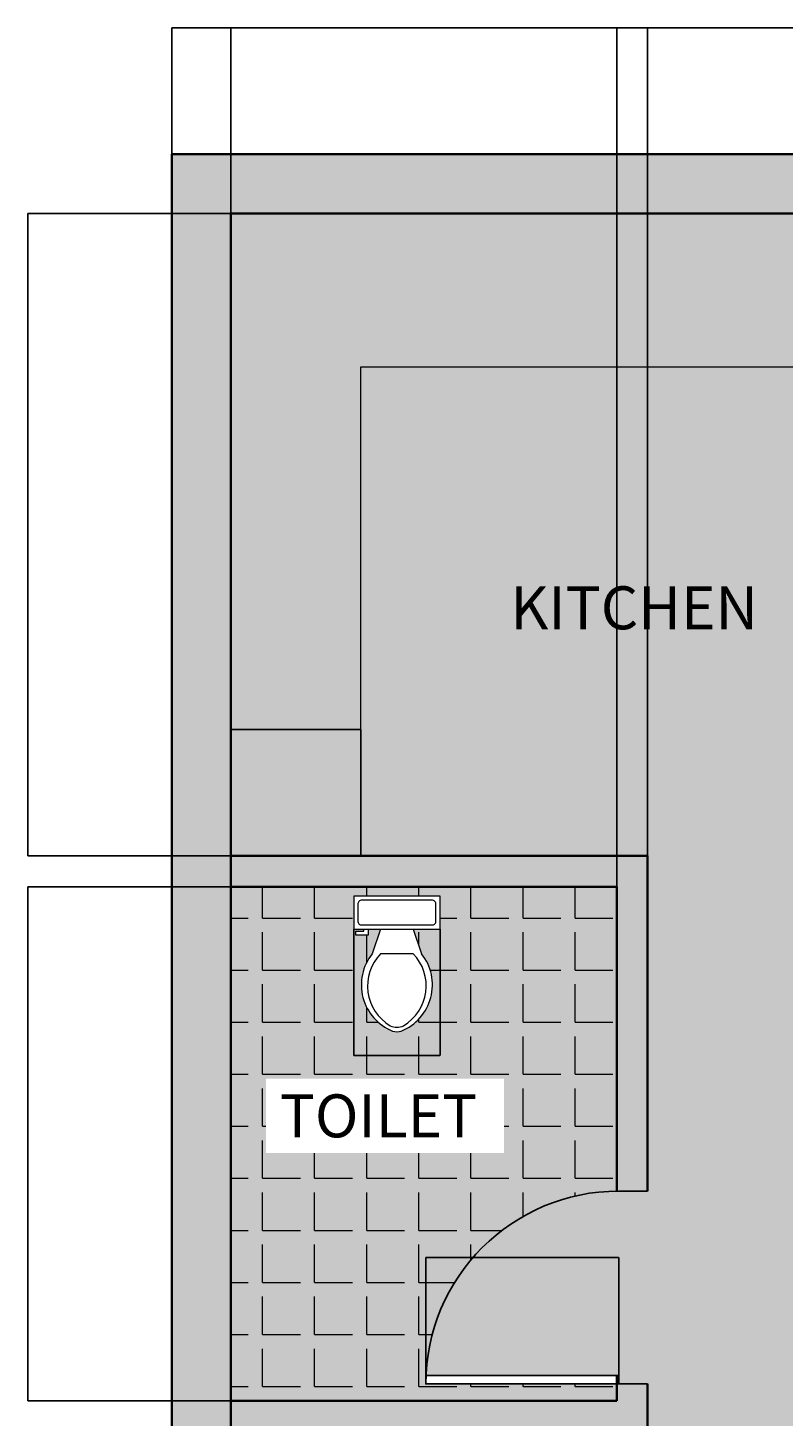
# Model space of a CAD drawing. Units: millimetres. Extents: x 1166 to 16630, y -7192 to 2820.
# Tile 5 of 8: x 1166 to 4103, y -2583 to 2820. Entities that reach past the tile are written whole.
import ezdxf

# ---------------------------------------------------------------- set-up
doc = ezdxf.new("R2010")
doc.units = ezdxf.units.MM
for name, color, linetype, lineweight in [('A-ANNO-DIMS', 2, 'Continuous', 18), ('A-AREA-IDEN', 7, 'Continuous', 18), ('A-DOOR', 4, 'Continuous', 25), ('A-FLOR-CASE', 8, 'Continuous', 18), ('A-FLOR-FIXT', 8, 'Continuous', 18), ('A-FLOR-PATT', 8, 'Continuous', 13), ('A-WALL', 7, 'Continuous', 35)]:
    doc.layers.add(name, color=color, linetype=linetype, lineweight=lineweight)
for name, color, linetype, lineweight, true_color in [('A-FLOR-CASE-PATT', 9, 'Continuous', 13, 0xc7c8ca), ('A-FLOR-FNSH-PATT', 254, 'Continuous', 13, 0xfeeab9), ('A-WALL-PATT', 254, 'Continuous', 13, 0xcecce6)]:
    doc.layers.add(name, color=color, linetype=linetype, lineweight=lineweight, true_color=true_color)
doc.styles.get("Standard").update_dxf_attribs({"font": 'arial.ttf'})
doc.dimstyles.get("Standard").update_dxf_attribs({"dimtxt": 0.18, "dimasz": 0.18, "dimexe": 0.18, "dimexo": 0.0625, "dimgap": 0.09, "dimtad": 0, "dimtih": 1, "dimtoh": 1, "dimdec": 4, "dimzin": 0, "dimdsep": 46, "dimtxsty": 'Standard', "dimcen": 0.09, "dimadec": 0, "dimazin": 0, "dimtfac": 1, "dimtdec": 4, "dimtofl": 0, "dimtmove": 0, "dimatfit": 3, "dimfxl": 1, "dimtolj": 1, "dimtzin": 0, "dimarcsym": 0})

# ---------------------------------------------------------------- blocks, each defined once
blk = doc.blocks.new('*U3')
for p, q in [((0, 0), (0, -6)), ((40, 0), (40, -6))]:
    blk.add_line(p, q)
blk.add_lwpolyline([(0, 0), (0, 40), (1.75, 40), (1.75, 0)], close=True)
blk.add_arc((0, 0), 40, 0, 90)
blk = doc.blocks.new('*U8')
for p, q in [((9.5, -6), (9.5, -2)), ((-10, -8.5), (-8, -8.5)), ((-10, -9.5), (-10, -8.5)), ((-7, -9.5), (-10, -9.5)), ((-8, -8.5), (-8, -8)), ((-7, -8), (-7, -9.5)), ((-4, -8), (-6, -14)), ((4, -8), (6, -14)), ((4, -14), (-4, -14))]:
    blk.add_line(p, q)
blk.add_lwpolyline([(10.5, -8), (10.5, 0), (-10.5, 0), (-10.5, -8)], close=True)
for points in [[(-9.5, -2), (-9.5, -6)], [(8.5, -1), (-8.5, -1)], [(-8.5, -7), (8.5, -7)]]:
    blk.add_lwpolyline(points)
for centre, radius, start, end in [((-8.62, -1.88), 0.884, 81.8699, 188.1301), ((8.62, -1.88), 0.884, 351.8699, 98.1301), ((-8.62, -6.12), 0.884, 171.8699, 278.1301), ((8.62, -6.12), 0.884, 261.8699, 8.1301), ((3.52, -21.58), 12.17, 141.4691, 247.9714), ((4.2, -21.82), 11.33, 136.3677, 238.9468), ((-3.52, -21.58), 12.17, 292.0284, 38.5307), ((-4.2, -21.82), 11.33, 301.053, 43.6321), ((0, -27.88), 4, 245.7318, 294.2682), ((0, -29), 4, 254.8605, 285.1395)]:
    blk.add_arc(centre, radius, start, end)
blk = doc.blocks.new('*D23')
at = {"layer": 'A-ANNO-DIMS', "color": 0, "lineweight": -2, "transparency": 16777216}
for p, q in [((1725.9, 2327.5), (1725.9, 2819.6)), ((1726.1, 2819.5), (4725.6, 2819.5)), ((7725.8, 2819.5), (4726.3, 2819.5)), ((7725.9, 2327.5), (7725.9, 2819.6))]:
    blk.add_line(p, q, dxfattribs=at)
at = {"layer": 'A-ANNO-DIMS', "color": 0, "transparency": 16777216}
for points in [[(1726.1, 2819.5), (1726.1, 2819.4), (1725.9, 2819.5)], [(7725.8, 2819.5), (7725.8, 2819.4), (7725.9, 2819.5)]]:
    blk.add_solid(points, dxfattribs=at)
at = {"layer": 'Defpoints', "color": 0, "transparency": 16777216}
for p in [(7725.9, 2819.5), (1725.9, 2327.5), (7725.9, 2327.5)]:
    blk.add_point(p, dxfattribs=at)
at = {"layer": 'A-ANNO-DIMS', "color": 0, "transparency": 16777216, "insert": (4725.9, 2819.5), "char_height": 0.18, "attachment_point": 5}
blk.add_mtext('\\A1;6000', dxfattribs=at)
blk = doc.blocks.new('*D25')
at = {"layer": 'A-ANNO-DIMS', "color": 0, "lineweight": -2, "transparency": 16777216}
for p, q in [((1955.939441, 2097.524735), (1955.939441, 2819.642235)), ((1956.119441, 2819.462235), (3310.579441, 2819.462235)), ((4665.759441, 2819.462235), (3311.299441, 2819.462235)), ((4665.939441, 2097.524735), (4665.939441, 2819.642235))]:
    blk.add_line(p, q, dxfattribs=at)
at = {"layer": 'A-ANNO-DIMS', "color": 0, "transparency": 16777216}
for points in [[(1956.119441, 2819.492235), (1956.119441, 2819.432235), (1955.939441, 2819.462235)], [(4665.759441, 2819.492235), (4665.759441, 2819.432235), (4665.939441, 2819.462235)]]:
    blk.add_solid(points, dxfattribs=at)
at = {"layer": 'Defpoints', "color": 0, "transparency": 16777216}
for p in [(4665.939441, 2819.462235), (1955.939441, 2097.462235), (4665.939441, 2097.462235)]:
    blk.add_point(p, dxfattribs=at)
at = {"layer": 'A-ANNO-DIMS', "color": 0, "transparency": 16777216, "insert": (3310.939441, 2819.462235), "char_height": 0.18, "attachment_point": 5}
blk.add_mtext('\\A1;2710', dxfattribs=at)
blk = doc.blocks.new('*D27')
at = {"layer": 'A-ANNO-DIMS', "color": 0, "lineweight": -2, "transparency": 16777216}
for p, q in [((1955.9, 2097.5), (1165.9, 2097.5)), ((1166.1, 2097.3), (1166.1, 847.6)), ((1166.1, -402.4), (1166.1, 847.3)), ((1955.9, -402.5), (1165.9, -402.5))]:
    blk.add_line(p, q, dxfattribs=at)
at = {"layer": 'A-ANNO-DIMS', "color": 0, "transparency": 16777216}
for points in [[(1166.1, 2097.3), (1166.1, 2097.3), (1166.1, 2097.5)], [(1166.1, -402.4), (1166.1, -402.4), (1166.1, -402.5)]]:
    blk.add_solid(points, dxfattribs=at)
at = {"layer": 'Defpoints', "color": 0, "transparency": 16777216}
for p in [(1166.1, 2097.5), (1955.9, 2097.5), (1955.9, -402.5)]:
    blk.add_point(p, dxfattribs=at)
at = {"layer": 'A-ANNO-DIMS', "color": 0, "transparency": 16777216, "insert": (1166.1, 847.5), "char_height": 0.18, "attachment_point": 5}
blk.add_mtext('\\A1;2500', dxfattribs=at)
blk = doc.blocks.new('*D28')
at = {"layer": 'A-ANNO-DIMS', "color": 0, "lineweight": -2, "transparency": 16777216}
for p, q in [((1955.9, -522.5), (1955.9, 2819.6)), ((1956.1, 2819.5), (2705.6, 2819.5)), ((3455.8, 2819.5), (2706.3, 2819.5)), ((3455.9, -522.5), (3455.9, 2819.6))]:
    blk.add_line(p, q, dxfattribs=at)
at = {"layer": 'A-ANNO-DIMS', "color": 0, "transparency": 16777216}
for points in [[(1956.1, 2819.5), (1956.1, 2819.4), (1955.9, 2819.5)], [(3455.8, 2819.5), (3455.8, 2819.4), (3455.9, 2819.5)]]:
    blk.add_solid(points, dxfattribs=at)
at = {"layer": 'Defpoints', "color": 0, "transparency": 16777216}
for p in [(3455.9, 2819.5), (1955.9, -522.5), (3455.9, -522.5)]:
    blk.add_point(p, dxfattribs=at)
at = {"layer": 'A-ANNO-DIMS', "color": 0, "transparency": 16777216, "insert": (2705.9, 2819.5), "char_height": 0.18, "attachment_point": 5}
blk.add_mtext('\\A1;1500', dxfattribs=at)
blk = doc.blocks.new('*D29')
at = {"layer": 'A-ANNO-DIMS', "color": 0, "lineweight": -2, "transparency": 16777216}
for p, q in [((1955.9, -522.5), (1165.9, -522.5)), ((1166.1, -522.7), (1166.1, -1522.4)), ((1166.1, -2522.4), (1166.1, -1522.7)), ((1955.9, -2522.5), (1165.9, -2522.5))]:
    blk.add_line(p, q, dxfattribs=at)
at = {"layer": 'A-ANNO-DIMS', "color": 0, "transparency": 16777216}
for points in [[(1166.1, -522.7), (1166.1, -522.7), (1166.1, -522.5)], [(1166.1, -2522.4), (1166.1, -2522.4), (1166.1, -2522.5)]]:
    blk.add_solid(points, dxfattribs=at)
at = {"layer": 'Defpoints', "color": 0, "transparency": 16777216}
for p in [(1955.9, -522.5), (1166.1, -2522.5), (1955.9, -2522.5)]:
    blk.add_point(p, dxfattribs=at)
at = {"layer": 'A-ANNO-DIMS', "color": 0, "transparency": 16777216, "insert": (1166.1, -1522.5), "char_height": 0.18, "attachment_point": 5}
blk.add_mtext('\\A1;2000', dxfattribs=at)
blk = doc.blocks.new('*D35')
at = {"layer": 'A-ANNO-DIMS', "color": 0, "lineweight": -2, "transparency": 16777216}
for p, q in [((2713.4, -2456.6), (2713.4, -1964.5)), ((2713.6, -1964.6), (3088.2, -1964.6)), ((3463.3, -1964.6), (3088.7, -1964.6)), ((3463.4, -2456.6), (3463.4, -1964.5))]:
    blk.add_line(p, q, dxfattribs=at)
at = {"layer": 'A-ANNO-DIMS', "color": 0, "transparency": 16777216}
for points in [[(2713.6, -1964.6), (2713.6, -1964.7), (2713.4, -1964.6)], [(3463.3, -1964.6), (3463.3, -1964.7), (3463.4, -1964.6)]]:
    blk.add_solid(points, dxfattribs=at)
at = {"layer": 'Defpoints', "color": 0, "transparency": 16777216}
for p in [(3463.4, -1964.6), (2713.4, -2456.6), (3463.4, -2456.6)]:
    blk.add_point(p, dxfattribs=at)
at = {"layer": 'A-ANNO-DIMS', "color": 0, "transparency": 16777216, "insert": (3088.4, -1964.6), "char_height": 0.18, "attachment_point": 5}
blk.add_mtext('\\A1;750', dxfattribs=at)
blk = doc.blocks.new('*D37')
at = {"layer": 'A-ANNO-DIMS', "color": 0, "lineweight": -2, "transparency": 16777216}
for p, q in [((3455.9, -1706.6), (3455.9, 2819.6)), ((3456.1, 2819.5), (3515.7, 2819.5)), ((3575.8, 2819.5), (3516.2, 2819.5)), ((3575.9, -1706.6), (3575.9, 2819.6))]:
    blk.add_line(p, q, dxfattribs=at)
at = {"layer": 'A-ANNO-DIMS', "color": 0, "transparency": 16777216}
for points in [[(3456.1, 2819.5), (3456.1, 2819.4), (3455.9, 2819.5)], [(3575.8, 2819.5), (3575.8, 2819.4), (3575.9, 2819.5)]]:
    blk.add_solid(points, dxfattribs=at)
at = {"layer": 'Defpoints', "color": 0, "transparency": 16777216}
for p in [(3575.9, 2819.5), (3455.9, -1706.7), (3575.9, -1706.6)]:
    blk.add_point(p, dxfattribs=at)
at = {"layer": 'A-ANNO-DIMS', "color": 0, "transparency": 16777216, "insert": (3515.9, 2819.5), "char_height": 0.18, "attachment_point": 5}
blk.add_mtext('\\A1;120', dxfattribs=at)
blk = doc.blocks.new('*D41')
at = {"layer": 'A-ANNO-DIMS', "color": 0, "lineweight": -2, "transparency": 16777216}
for p, q in [((1955.9, -402.5), (1955.9, 89.6)), ((1956.1, 89.5), (2207.8, 89.5)), ((2460.4, 89.5), (2208.6, 89.5)), ((2460.5, -402.5), (2460.5, 89.6))]:
    blk.add_line(p, q, dxfattribs=at)
at = {"layer": 'A-ANNO-DIMS', "color": 0, "transparency": 16777216}
for points in [[(1956.1, 89.5), (1956.1, 89.4), (1955.9, 89.5)], [(2460.4, 89.5), (2460.4, 89.4), (2460.5, 89.5)]]:
    blk.add_solid(points, dxfattribs=at)
at = {"layer": 'Defpoints', "color": 0, "transparency": 16777216}
for p in [(2460.5, 89.5), (1955.9, -402.5), (2460.5, -402.5)]:
    blk.add_point(p, dxfattribs=at)
at = {"layer": 'A-ANNO-DIMS', "color": 0, "transparency": 16777216, "insert": (2208.2, 89.5), "char_height": 0.18, "attachment_point": 5}
blk.add_mtext('\\A1;504.6', dxfattribs=at)
blk = doc.blocks.new('*D43')
at = {"layer": 'A-ANNO-DIMS', "color": 0, "lineweight": -2, "transparency": 16777216}
for p, q in [((2433.1, -687.1), (2433.1, -1179.2)), ((2768.8, -687.1), (2768.8, -1179.2)), ((2433.3, -1179), (2600.5, -1179)), ((2768.6, -1179), (2601.4, -1179))]:
    blk.add_line(p, q, dxfattribs=at)
at = {"layer": 'A-ANNO-DIMS', "color": 0, "transparency": 16777216}
for points in [[(2433.3, -1179), (2433.3, -1179.1), (2433.1, -1179)], [(2768.6, -1179), (2768.6, -1179.1), (2768.8, -1179)]]:
    blk.add_solid(points, dxfattribs=at)
at = {"layer": 'Defpoints', "color": 0, "transparency": 16777216}
for p in [(2433.1, -687), (2768.8, -687), (2433.1, -1179)]:
    blk.add_point(p, dxfattribs=at)
at = {"layer": 'A-ANNO-DIMS', "color": 0, "transparency": 16777216, "insert": (2601, -1179), "char_height": 0.18, "attachment_point": 5}
blk.add_mtext('\\A1;335.66', dxfattribs=at)

msp = doc.modelspace()

# ---------------------------------------------------------------- hatches: boundary and pattern name
at = {"layer": 'A-FLOR-CASE-PATT'}
h = msp.add_hatch(color=256, dxfattribs=at)
h.dxf.hatch_style = 1
h.paths.add_polyline_path([(2460.545, 1500.697), (4665.939, 1500.697), (4665.939, 2097.462), (1955.939, 2097.462), (1955.939, -402.538), (2460.545, -402.538)])
at = {"layer": 'A-FLOR-FNSH-PATT', "transparency": 33554523}
h = msp.add_hatch(color=256, dxfattribs=at)
h.dxf.hatch_style = 1
h.paths.add_polyline_path([(7725.939, 2327.462), (1725.939, 2327.462), (1725.939, -5672.538), (5309.615, -5672.538), (5309.615, -2642.538), (5189.615, -2642.538), (5189.615, -5442.538), (1955.939, -5442.538), (1955.939, 2097.462), (4665.939, 2097.462), (4665.939, 150.2), (4815.939, 150.2, -0.40145271), (5814.982, -806.05), (5815.939, -806.05), (5815.939, -849.8), (4815.939, -849.8), (4785.939, -849.8), (4785.939, -902.538), (7495.939, -902.538), (7495.939, -2522.538), (4884.014, -2522.538), (4884.014, -2642.538), (7725.939, -2642.538)], flags=17)
h.paths.add_polyline_path([(6066.077, 618.421), (6066.077, 1624.186), (7407.098, 1624.186), (7407.098, 618.421)], flags=16)
h.paths.add_polyline_path([(4979.212, 660.219), (4799.278, 660.219), (4799.278, 780.174), (4789.282, 790.171), (4789.282, 870.141), (4799.278, 880.137), (4799.278, 1259.997), (4979.212, 1259.997), (4979.212, 1230.008), (4989.208, 1230.008), (4989.208, 1110.052), (4979.212, 1110.052), (4979.212, 1100.056), (4989.208, 1100.056), (4989.208, 980.1), (4979.212, 980.1), (4979.212, 950.111), (4989.208, 950.111), (4989.208, 940.115, -0.09090909), (4989.208, 720.196), (4989.208, 710.2), (4979.212, 710.2)], flags=16)
h.paths.add_polyline_path([(4974.214, 665.217), (4804.276, 665.217), (4804.276, 1254.999), (4974.214, 1254.999)], flags=0)
h.paths.add_polyline_path([(6910.92, 618.421), (6910.92, 873.215), (7165.714, 873.215), (7165.714, 1490.084), (7386.983, 1490.084), (7386.983, 1141.419), (7165.714, 1141.419), (7165.714, 1101.188), (7386.983, 1101.188), (7386.983, 752.523), (7132.189, 752.523), (7132.189, 839.689)], flags=16)
h.paths.add_polyline_path([(4815.939, 150.2), (4665.939, 150.2), (4665.939, 1500.697), (2460.545, 1500.697), (2460.545, -402.538), (3575.939, -402.538), (3575.939, -1706.64), (3463.439, -1706.64, 0.40145271), (2714.158, -2423.828), (3463.439, -2423.828), (3463.439, -2456.64), (3455.939, -2522.538), (3455.939, -2456.64), (2713.439, -2456.64), (2713.439, -2423.828), (2714.158, -2423.828, -0.39855266), (3455.939, -1706.678), (3455.939, -1706.64), (3575.939, -1706.64), (3575.939, -402.538), (2460.545, -402.538), (2460.545, 1500.697), (4665.939, 1500.697), (4665.939, 150.2), (4785.939, 150.2), (4785.939, 2097.462), (7495.939, 2097.462), (7495.939, -2522.538), (4884.014, -2522.538), (4884.014, -2642.538), (7725.939, -2642.538), (7725.939, 2327.462), (1725.939, 2327.462), (1725.939, -5672.538), (5309.615, -5672.538), (5309.615, -2642.538), (4884.014, -2642.538), (4884.014, -2522.538), (4884.014, -1822.538), (4665.939, -1822.538), (4665.939, -1722.538), (4665.939, -1022.538), (4665.939, -849.8), (4815.939, -849.8), (4815.939, -806.05), (5814.982, -806.05, 0.40145271)])
h.paths.add_polyline_path([(1955.939, -4323.626), (1965.936, -4313.63), (1965.936, -3933.77), (2145.869, -3933.77), (2145.869, -3963.759), (2155.866, -3963.759), (2155.866, -4083.715), (2145.869, -4083.715), (2145.869, -4093.711), (2155.866, -4093.711), (2155.866, -4213.667), (2145.869, -4213.667), (2145.869, -4243.656), (2155.866, -4243.656), (2155.866, -4253.652, -0.09090909), (2155.866, -4473.571), (2155.866, -4483.567), (2145.869, -4483.567), (2145.869, -4533.549), (1965.936, -4533.549), (1965.936, -4413.593), (1955.939, -4403.597)], flags=16)
h.paths.add_polyline_path([(3017.672, -1268.685), (3017.672, -1558.932), (2092.538, -1558.932), (2092.538, -1268.685)], flags=16)
h.paths.add_polyline_path([(2768.799, -687.028), (2664.904, -687.028), (2696.871, -782.93, -0.50132349), (2617.667, -1084.405, -0.13289091), (2584.271, -1084.405, -0.50131678), (2505.065, -782.933), (2537.033, -687.028), (2489.082, -687.028), (2489.082, -711.004), (2441.13, -711.004), (2441.13, -687.028), (2433.138, -687.028), (2433.138, -559.158), (2768.799, -559.158)], flags=16)
h.paths.add_polyline_path([(2752.815, -655.061, -0.41421356), (2740.827, -671.045), (2465.106, -671.045, -0.41421356), (2449.122, -659.057), (2449.122, -591.126, -0.41421356), (2461.11, -575.142), (2736.831, -575.142, -0.41421356), (2752.815, -587.13)], flags=0)
h.paths.add_polyline_path([(2627.247, -1063.016, -0.21500378), (2574.691, -1063.016, -0.48007965), (2537.034, -782.931), (2664.904, -782.931, -0.4800795)], flags=0)
h.paths.add_polyline_path([(4505.634, -3647.875), (4977.863, -3647.875, -0.19047621), (4977.864, -5173.541), (4505.634, -5173.541), (4505.634, -5064.565), (4533.929, -5064.565), (4533.929, -3756.851), (4505.634, -3756.851)], flags=16)
h.paths.add_polyline_path([(4880.114, -4192.756), (5003.372, -4192.756, -0.04962821), (5003.372, -4628.66), (4880.114, -4628.66)], flags=0)
h.paths.add_polyline_path([(2140.871, -3938.769), (2140.871, -4528.551), (1970.934, -4528.551), (1970.934, -3938.769)], flags=0)
h.paths.add_polyline_path([(7495.939, -1022.538), (6660.699, -1022.538), (6660.699, -1722.538, -0.21291191), (6697.901, -1739.132)], flags=16)
h.paths.add_polyline_path([(7495.939, -1022.538), (6697.901, -1739.132, -0.18498743), (6710.699, -1772.538), (7495.939, -1772.538)], flags=16)
h.paths.add_polyline_path([(7495.939, -1772.538), (6710.699, -1772.538, -0.18498743), (6697.901, -1805.944), (7495.939, -2522.538)], flags=16)
h.paths.add_polyline_path([(6697.901, -1805.944, -0.21291191), (6660.699, -1822.538), (6660.699, -2522.538), (7495.939, -2522.538)], flags=16)
h.paths.add_polyline_path([(6660.699, -1822.538), (6438.613, -1822.538), (6438.613, -2522.538), (6660.699, -2522.538)], flags=16)
h.paths.add_polyline_path([(6438.613, -1822.538), (6216.528, -1822.538), (6216.528, -2522.538), (6438.613, -2522.538)], flags=16)
h.paths.add_polyline_path([(6216.528, -1822.538), (5994.442, -1822.538), (5994.442, -2522.538), (6216.528, -2522.538)], flags=16)
h.paths.add_polyline_path([(5994.442, -1822.538), (5772.357, -1822.538), (5772.357, -2522.538), (5994.442, -2522.538)], flags=16)
h.paths.add_polyline_path([(5550.271, -1822.538), (5328.185, -1822.538), (5328.185, -2522.538), (5550.271, -2522.538)], flags=16)
h.paths.add_polyline_path([(5328.185, -1822.538), (5106.1, -1822.538), (5106.1, -2522.538), (5328.185, -2522.538)], flags=16)
h.paths.add_polyline_path([(5106.1, -1822.538), (4884.014, -1822.538), (4884.014, -2522.538), (5106.1, -2522.538)], flags=16)
h.paths.add_polyline_path([(4884.014, -1022.538), (4665.939, -1022.538), (4665.939, -1722.538), (4884.014, -1722.538)], flags=16)
h.paths.add_polyline_path([(5106.1, -1022.538), (4884.014, -1022.538), (4884.014, -1722.538), (5106.1, -1722.538)], flags=16)
h.paths.add_polyline_path([(5550.271, -1022.538), (5328.185, -1022.538), (5328.185, -1722.538), (5550.271, -1722.538)], flags=16)
h.paths.add_polyline_path([(5328.185, -1022.538), (5106.1, -1022.538), (5106.1, -1722.538), (5328.185, -1722.538)], flags=16)
h.paths.add_polyline_path([(5772.357, -1022.538), (5550.271, -1022.538), (5550.271, -1722.538), (5772.357, -1722.538)], flags=16)
h.paths.add_polyline_path([(5994.442, -1022.538), (5772.357, -1022.538), (5772.357, -1722.538), (5994.442, -1722.538)], flags=16)
h.paths.add_polyline_path([(6216.528, -1022.538), (5994.442, -1022.538), (5994.442, -1722.538), (6216.528, -1722.538)], flags=16)
h.paths.add_polyline_path([(6660.699, -1022.538), (6438.613, -1022.538), (6438.613, -1722.538), (6660.699, -1722.538)], flags=16)
h.paths.add_polyline_path([(6438.613, -1022.538), (6216.528, -1022.538), (6216.528, -1722.538), (6438.613, -1722.538)], flags=16)
h.paths.add_polyline_path([(5772.357, -1822.538), (5550.271, -1822.538), (5550.271, -2522.538), (5772.357, -2522.538)], flags=16)
h.paths.add_polyline_path([(6660.699, -1722.538), (6438.613, -1722.538), (4665.939, -1722.538), (4665.939, -1822.538), (6660.699, -1822.538, 0.21291191), (6697.901, -1805.944, 0.64892437)], flags=16)
h.paths.add_polyline_path([(5860.25, -44.006), (7154.504, -44.006), (7154.504, 215.689), (5860.25, 215.689)], flags=24)
h.paths.add_polyline_path([(2102.336, -1543.656), (3007.075, -1543.656), (3007.075, -1283.961), (2102.336, -1283.961)], flags=8)
h.paths.add_polyline_path([(2887.503, -4248.68), (3740.372, -4248.68), (3740.372, -3989.156), (2887.503, -3989.156)], flags=24)
h.paths.add_polyline_path([(2999.436, 433.054), (4111.829, 433.054), (4111.829, 692.578), (2999.436, 692.578)], flags=24)
at = {"layer": 'A-FLOR-FNSH-PATT', "transparency": 33554590}
h = msp.add_hatch(color=256, dxfattribs=at)
h.dxf.hatch_style = 1
h.paths.add_polyline_path([(5309.615, -2642.538), (5309.615, -6304.141), (7725.939, -6304.141), (7725.939, -5672.538), (7725.939, -2642.538)])
edge = h.paths.add_edge_path(flags=16)
edge.add_ellipse((-448.972, -3645.43), major_axis=(-7430.723, 0), ratio=0.84230387, start_angle=182.1799503, end_angle=183.6504276, ccw=False)
edge.add_line((6974.174, -3362.862), (6984.716, -3362.862))
edge.add_ellipse((6982.281, -3380.397), major_axis=(-20.817, 0), ratio=0.84230387, start_angle=180, end_angle=270, ccw=False)
edge.add_line((7003.098, -3380.397), (7003.098, -3722.916))
edge.add_ellipse((6982.281, -3720.865), major_axis=(20.817, 0), ratio=0.84230387, start_angle=270, end_angle=360, ccw=False)
edge.add_ellipse((-142030.923, -3973.064), major_axis=(149013.204, 0), ratio=0.8423038695, start_angle=-0.38386678, end_angle=0.09022909, ccw=False)
edge.add_line((6977.567, -4971.397), (6984.47, -4971.397))
edge.add_ellipse((6982.281, -4988.932), major_axis=(20.817, 0), ratio=0.84230387, start_angle=0, end_angle=90, ccw=False)
edge.add_line((7003.098, -4988.932), (7003.098, -5331.243))
edge.add_ellipse((6982.281, -5329.4), major_axis=(-20.817, 0), ratio=0.84230387, start_angle=90, end_angle=180, ccw=False)
edge.add_line((6982.281, -5346.934), (6973.354, -5346.934))
edge.add_ellipse((-142030.923, -3973.064), major_axis=(149013.204, 0), ratio=0.8423038695, start_angle=-0.6186432, end_angle=-0.52827147, ccw=False)
edge.add_ellipse((6960.189, -5606.903), major_axis=(-31.226, 0), ratio=0.84230387, start_angle=179.371763, end_angle=248.464757, ccw=False)
edge.add_ellipse((-142041.332, -3973.064), major_axis=(-149045.372, 0), ratio=0.8423038661, start_angle=179.35344592, end_angle=179.3717628, ccw=False)
edge.add_ellipse((6916.87, -5654.054), major_axis=(-73.802, 0), ratio=0.84230387, start_angle=90, end_angle=179.353446, ccw=False)
edge.add_line((6916.87, -5716.218), (5995.23, -5716.218))
edge.add_ellipse((5995.23, -5654.054), major_axis=(73.802, 0), ratio=0.84230387, start_angle=180.646554, end_angle=270, ccw=False)
edge.add_ellipse((154953.432, -3973.064), major_axis=(-149045.372, 0), ratio=0.8423038697, start_angle=0.62823722, end_angle=0.6465541, ccw=False)
edge.add_ellipse((5951.911, -5606.903), major_axis=(31.226, 0), ratio=0.84230387, start_angle=111.535244, end_angle=180.628237, ccw=False)
edge.add_ellipse((154943.023, -3973.064), major_axis=(-149013.204, 0), ratio=0.8423038695, start_angle=0.52827147, end_angle=0.6465541, ccw=False)
edge.add_line((5938.746, -5346.934), (5927.384, -5346.934))
edge.add_ellipse((5929.819, -5329.4), major_axis=(20.817, 0), ratio=0.84230387, start_angle=180, end_angle=270, ccw=False)
edge.add_line((5909.002, -5329.4), (5909.002, -4986.881))
edge.add_ellipse((5929.819, -4988.932), major_axis=(-20.817, 0), ratio=0.84230387, start_angle=-90, end_angle=0, ccw=False)
edge.add_line((5929.819, -4971.397), (5934.533, -4971.397))
edge.add_ellipse((154943.023, -3973.064), major_axis=(-149013.204, 0), ratio=0.8423038695, start_angle=-0.09022909, end_angle=0.38386678, ccw=False)
edge.add_ellipse((5929.819, -3720.865), major_axis=(-20.817, 0), ratio=0.84230387, start_angle=0, end_angle=90, ccw=False)
edge.add_line((5909.002, -3720.865), (5909.002, -3378.346))
edge.add_ellipse((5929.819, -3380.397), major_axis=(20.817, 0), ratio=0.84230387, start_angle=90, end_angle=180, ccw=False)
edge.add_line((5929.819, -3362.862), (5937.926, -3362.862))
edge.add_ellipse((13361.072, -3645.43), major_axis=(7430.723, 0), ratio=0.84230387, start_angle=176.3495724, end_angle=177.8200497, ccw=False)
edge.add_ellipse((6843.239, -6808.261), major_axis=(4407.333, 0), ratio=0.84230387, start_angle=102.125966, end_angle=103.780529, ccw=False)
edge.add_ellipse((6843.239, -6711.831), major_axis=(4294.728, 0), ratio=0.84230387, start_angle=100.209539, end_angle=102.444627, ccw=False)
edge.add_ellipse((5718.978, -189.342), major_axis=(-3530.283, 0), ratio=0.84230387, start_angle=99.256566, end_angle=102.554933)
edge.add_line((6369.843, -3111.939), (6452.047, -3066.483))
edge.add_ellipse((6456.05, -3074.757), major_axis=(-10.409, 0), ratio=0.84230387, start_angle=270, end_angle=307.93313, ccw=False)
edge.add_ellipse((6456.05, -3074.757), major_axis=(-10.409, 0), ratio=0.84230387, start_angle=232.06687, end_angle=270, ccw=False)
edge.add_line((6461.762, -3067.428), (6542.257, -3111.939))
edge.add_ellipse((7193.122, -189.342), major_axis=(3530.283, 0), ratio=0.84230387, start_angle=257.445067, end_angle=260.743434)
edge.add_ellipse((6068.861, -6711.831), major_axis=(4294.728, 0), ratio=0.84230387, start_angle=77.555373, end_angle=79.790461, ccw=False)
edge.add_ellipse((6068.861, -6808.261), major_axis=(-4407.333, 0), ratio=0.84230387, start_angle=256.219471, end_angle=257.874034, ccw=False)
edge = h.paths.add_edge_path(flags=0)
edge.add_ellipse((5799.636, -3484.806), major_axis=(790.133, 0), ratio=0.84230387, start_angle=0, end_angle=29.43857, ccw=False)
edge.add_line((6589.77, -3484.806), (6589.77, -3517.866))
edge.add_line((6589.77, -3517.866), (6615.397, -3517.866))
edge.add_ellipse((6612.95, -3526.633), major_axis=(10.409, 0), ratio=0.84230387, start_angle=45.519789, end_angle=90, ccw=False)
edge.add_line((6619.584, -3519.877), (6697.577, -3574.216))
edge.add_line((6697.577, -3574.216), (6697.577, -3782.552))
edge.add_ellipse((6643.673, -3780.461), major_axis=(5.016, 89.187), ratio=0.60383358, start_angle=106.342592, end_angle=270.997986, ccw=False)
edge.add_line((6589.77, -3793.028), (6589.77, -3484.806))
edge.add_ellipse((5799.636, -3484.806), major_axis=(790.133, 0), ratio=0.84230387, start_angle=0, end_angle=29.43857)
edge.add_ellipse((7112.464, -3484.806), major_axis=(-790.133, 0), ratio=0.84230387, start_angle=-29.43857, end_angle=0)
edge.add_line((6322.33, -3484.806), (6322.33, -3793.028))
edge.add_ellipse((6268.427, -3780.461), major_axis=(-5.016, 89.187), ratio=0.60383358, start_angle=89.002014, end_angle=253.657408, ccw=False)
edge.add_line((6214.523, -3782.552), (6214.523, -3574.216))
edge.add_line((6214.523, -3574.216), (6294.401, -3518.564))
edge.add_ellipse((6299.15, -3526.633), major_axis=(10.409, 0), ratio=0.84230387, start_angle=90, end_angle=134.480211, ccw=False)
edge.add_line((6299.15, -3517.866), (6322.33, -3517.866))
edge.add_line((6322.33, -3517.866), (6322.33, -3484.806))
edge.add_ellipse((7112.464, -3484.806), major_axis=(-790.133, 0), ratio=0.84230387, start_angle=-29.43857, end_angle=0, ccw=False)
edge = h.paths.add_edge_path(flags=0)
edge.add_line((6899.672, -4051.113), (6868.937, -4281.474))
edge.add_ellipse((6495.43, -5170.363), major_axis=(1119.455, 0), ratio=0.84230387, start_angle=67.208085, end_angle=85.12993)
edge.add_line((6575.565, -4229.86), (6336.535, -4229.86))
edge.add_ellipse((6416.67, -5170.363), major_axis=(1119.455, 0), ratio=0.84230387, start_angle=94.87007, end_angle=112.791915)
edge.add_line((6043.163, -4281.474), (6012.428, -4051.113))
edge.add_ellipse((6380.264, -4969.144), major_axis=(1150.303, 0), ratio=0.84230387, start_angle=94.277421, end_angle=111.834954, ccw=False)
edge.add_line((6307.939, -4002.156), (6604.161, -4002.156))
edge.add_ellipse((6531.836, -4969.144), major_axis=(-1150.303, 0), ratio=0.84230387, start_angle=248.165046, end_angle=265.722579, ccw=False)
edge = h.paths.add_edge_path(flags=0)
edge.add_ellipse((-142030.923, -3973.064), major_axis=(-148992.387, 0), ratio=0.8423038695, start_angle=179.62223581, end_angle=179.94440569, ccw=False)
edge.add_line((6956.9, -4955.389), (6903.068, -4744.03))
edge.add_ellipse((-45118.924, -4413.46), major_axis=(52023.473, 0), ratio=0.84230387, start_angle=-0.3640763, end_angle=0.1208974)
edge.add_line((6904.386, -4303.688), (6961.365, -4117.632))
edge = h.paths.add_edge_path(flags=0)
edge.add_line((5950.735, -4117.632), (6007.714, -4303.688))
edge.add_ellipse((58031.024, -4413.46), major_axis=(-52023.473, 0), ratio=0.84230387, start_angle=-0.1208974, end_angle=0.3640763)
edge.add_line((6009.031, -4744.03), (5955.2, -4955.389))
edge.add_ellipse((154943.023, -3973.064), major_axis=(-148992.387, 0), ratio=0.8423038696, start_angle=0.05559431, end_angle=0.37776419, ccw=False)
edge = h.paths.add_edge_path(flags=0)
edge.add_line((6868.937, -5013.198), (6868.937, -5277.993))
edge.add_ellipse((6456.05, -3571.079), major_axis=(2068.116, 0), ratio=0.84230387, start_angle=256.401865, end_angle=283.598135, ccw=False)
edge.add_line((6043.163, -5277.993), (6043.163, -5013.198))
edge.add_ellipse((6456.05, -3306.285), major_axis=(2068.116, 0), ratio=0.84230387, start_angle=256.401865, end_angle=283.598135)
edge = h.paths.add_edge_path(flags=0)
edge.add_ellipse((6827.303, -5415.313), major_axis=(-41.634, 0), ratio=0.84230387, start_angle=180, end_angle=270, ccw=False)
edge.add_line((6868.937, -5415.313), (6868.937, -5689.123))
edge.add_line((6868.937, -5689.123), (6043.163, -5689.123))
edge.add_line((6043.163, -5689.123), (6043.163, -5415.313))
edge.add_ellipse((6084.797, -5415.313), major_axis=(-41.634, 0), ratio=0.84230387, start_angle=-90, end_angle=0, ccw=False)
edge.add_line((6084.797, -5380.245), (6827.303, -5380.245))
h.paths.add_polyline_path([(3455.939, -522.538), (1955.939, -522.538), (1955.939, -2522.538), (3455.939, -2522.538), (3455.939, -2456.64), (2713.439, -2456.64), (2713.439, -2423.828), (2714.158, -2423.828, -0.39855266), (3455.939, -1706.678)])
h.paths.add_polyline_path([(2617.667, -1084.405, -0.13289091), (2584.271, -1084.405, -0.50131678), (2505.065, -782.933), (2537.033, -687.028), (2489.082, -687.028), (2489.082, -711.004), (2441.13, -711.004), (2441.13, -695.02), (2473.098, -695.02), (2473.098, -687.028), (2433.138, -687.028), (2433.138, -559.158), (2768.799, -559.158), (2768.799, -687.028), (2664.904, -687.028), (2696.871, -782.93, -0.50132349)], flags=16)
h.paths.add_polyline_path([(2627.247, -1063.016, -0.21500378), (2574.691, -1063.016, -0.48007965), (2537.034, -782.931), (2664.904, -782.931, -0.4800795)], flags=0)
h.paths.add_polyline_path([(2736.831, -671.045), (2465.106, -671.045, -0.50000012), (2449.122, -655.061), (2449.122, -591.126, -0.50000012), (2465.106, -575.142), (2736.831, -575.142, -0.50000012), (2752.815, -591.126), (2752.815, -655.061, -0.50000012)], flags=0)
h.paths.add_polyline_path([(5931.782, -6111.826), (7070.31, -6111.826), (7070.31, -5852.302), (5931.782, -5852.302)], flags=24)
h.paths.add_polyline_path([(2102.336, -1543.656), (3007.075, -1543.656), (3007.075, -1283.961), (2102.336, -1283.961)], flags=24)
at = {"layer": 'A-FLOR-PATT', "transparency": 33554564}
h = msp.add_hatch(dxfattribs=at)
h.set_pattern_fill('ANGLE', color=256, scale=29)
h.set_pattern_definition([(0, (-8657.52, -11987.85), (0, 202.565), [147.32, -55.245]), (90, (-8657.52, -11987.85), (-202.565, 1e-14), [147.32, -55.245])])
h.paths.add_polyline_path([(3455.939, -1706.678), (3455.939, -522.538), (1955.939, -522.538), (1955.939, -2522.538), (3455.939, -2522.538), (3455.939, -2456.64), (2713.439, -2456.64), (2713.439, -2423.828), (2714.158, -2423.828, -0.39855266)])
h.paths.add_polyline_path([(2584.271, -1084.405, -0.50131678), (2505.065, -782.933), (2537.033, -687.028), (2489.082, -687.028), (2489.082, -711.004), (2441.13, -711.004), (2441.13, -695.02), (2473.098, -695.02), (2473.098, -687.028), (2433.138, -687.028), (2433.138, -559.158), (2768.799, -559.158), (2768.799, -687.028), (2664.904, -687.028), (2696.871, -782.93, -0.50132349), (2617.667, -1084.405, -0.13289091)], flags=16)
h.paths.add_polyline_path([(2574.691, -1063.016, -0.48007965), (2537.034, -782.931), (2664.904, -782.931, -0.4800795), (2627.247, -1063.016, -0.21500378)], flags=0)
h.paths.add_polyline_path([(2465.106, -671.045, -0.50000012), (2449.122, -655.061), (2449.122, -591.126, -0.50000012), (2465.106, -575.142), (2736.831, -575.142, -0.50000012), (2752.815, -591.126), (2752.815, -655.061, -0.50000012), (2736.831, -671.045)], flags=0)
at = {"layer": 'A-WALL-PATT'}
h = msp.add_hatch(color=256, dxfattribs=at)
h.dxf.hatch_style = 1
h.paths.add_polyline_path([(1955.939, 2097.462), (4665.939, 2097.462), (4665.939, 150.2), (4785.939, 150.2), (4785.939, 2097.462), (7495.939, 2097.462), (7495.939, -2522.538), (4884.014, -2522.538), (4884.014, -2642.538), (7725.939, -2642.538), (7725.939, 2327.462), (1725.939, 2327.462), (1725.939, -5672.538), (5309.615, -5672.538), (5309.615, -2642.538), (5189.615, -2642.538), (5189.615, -5442.538), (1955.939, -5442.538)])
h.paths.add_polyline_path([(7495.939, -902.538), (4785.939, -902.538), (4785.939, -849.8), (4665.939, -849.8), (4665.939, -1022.538), (7495.939, -1022.538)], flags=17)
h.paths.add_polyline_path([(3575.939, -402.538), (1955.939, -402.538), (1955.939, -522.538), (3455.939, -522.538), (3455.939, -1706.64), (3575.939, -1706.64)], flags=17)
h.paths.add_polyline_path([(3575.939, -2456.64), (3455.939, -2456.64), (3455.939, -2522.538), (1955.939, -2522.538), (1955.939, -2642.538), (3575.939, -2642.538)], flags=17)

# ---------------------------------------------------------------- linework, layer by layer
at = {"layer": 'A-FLOR-CASE', "transparency": 33554559}
for p, q in [((2460.545, -402.538), (2460.545, 1500.697)), ((2460.545, 1500.697), (4665.939, 1500.697))]:
    msp.add_line(p, q, dxfattribs=at)
at = {"layer": 'A-WALL'}
for p, q in [((1955.939, -5442.538), (1955.939, 2097.462)), ((1955.939, 2097.462), (4665.939, 2097.462)), ((1955.939, -402.538), (3575.939, -402.538)), ((3575.939, -1706.64), (3575.939, -402.538)), ((1955.939, -522.538), (3455.939, -522.538)), ((3455.939, -1706.678), (3455.939, -522.538)), ((3455.939, -2522.538), (3455.939, -2423.828)), ((3575.939, -2642.538), (3575.939, -2456.64)), ((1955.939, -2522.538), (3455.939, -2522.538))]:
    msp.add_line(p, q, dxfattribs=at)
msp.add_lwpolyline([(5309.615, -5672.538), (1725.939, -5672.538), (1725.939, 2327.462), (7725.939, 2327.462), (7725.939, -5672.538)], dxfattribs=at)

# ---------------------------------------------------------------- block references
at = {"layer": 'A-DOOR', "xscale": 18.75, "yscale": 18.75, "zscale": 18.75, "rotation": 90}
msp.add_blockref('*U3', (3463.439, -2456.64), dxfattribs=at)
at = {"layer": 'A-FLOR-FIXT', "xscale": 15.98382298506819, "yscale": 15.98382298506819, "zscale": 15.98382298506819}
msp.add_blockref('*U8', (2600.968, -559.158), dxfattribs=at)

# ---------------------------------------------------------------- texts
at = {"layer": 'A-AREA-IDEN'}
msp.add_text('KITCHEN', height=167.3098, dxfattribs=at).set_placement((3042.69, 479.161))

# ---------------------------------------------------------------- dimensions: what is measured, and where the dimension line sits
at = {"layer": 'A-ANNO-DIMS'}
for base, p1, p2, override, picture, middle in [((7725.939, 2819.462), (1725.939, 2327.462), (7725.939, 2327.462), {"dimdec": 0, "dimlfac": 1, "dimrnd": 0, "dimzin": 0, "dimdsep": 46, "dimlunit": 2}, '*D23', (4725.939, 2819.462)), ((4665.939, 2819.462), (1955.939, 2097.462), (4665.939, 2097.462), {"dimdec": 0, "dimlfac": 1, "dimrnd": 0, "dimzin": 0, "dimdsep": 46, "dimlunit": 2}, '*D25', (3310.939, 2819.462)), ((3455.939, 2819.462), (1955.939, -522.538), (3455.939, -522.538), {"dimdec": 0, "dimlfac": 1, "dimrnd": 0, "dimzin": 0, "dimdsep": 46, "dimlunit": 2}, '*D28', (2705.939, 2819.462)), ((3575.939, 2819.462), (3455.939, -1706.678), (3575.939, -1706.64), {"dimdec": 0, "dimlfac": 1, "dimrnd": 0, "dimzin": 0, "dimdsep": 46, "dimlunit": 2}, '*D37', (3515.939, 2819.462)), ((2460.545, 89.462), (1955.939, -402.538), (2460.545, -402.538), {"dimdec": 1, "dimlfac": 1, "dimrnd": 0, "dimzin": 0, "dimdsep": 46, "dimlunit": 2}, '*D41', (2208.242, 89.462)), ((3463.439, -1964.64), (2713.439, -2456.64), (3463.439, -2456.64), {"dimdec": 0, "dimlfac": 1, "dimrnd": 0, "dimzin": 0, "dimdsep": 46, "dimlunit": 2}, '*D35', (3088.439, -1964.64))]:
    dim = msp.add_linear_dim(base=base, p1=p1, p2=p2, dimstyle='Standard', override=override, dxfattribs=at)
    dim.commit()
    dim.dimension.update_dxf_attribs({"geometry": picture, "text_midpoint": middle})
for base, p1, p2, angle, override, picture, middle in [((1166.088, 2097.462), (1955.939, -402.538), (1955.939, 2097.462), 90, {"dimdec": 0, "dimlfac": 1, "dimrnd": 0, "dimzin": 0, "dimdsep": 46, "dimlunit": 2}, '*D27', (1166.088, 847.462)), ((1166.088, -2522.538), (1955.939, -522.538), (1955.939, -2522.538), 90, {"dimdec": 0, "dimlfac": 1, "dimrnd": 0, "dimzin": 0, "dimdsep": 46, "dimlunit": 2}, '*D29', (1166.088, -1522.538)), ((2433.138, -1179.028), (2768.799, -687.028), (2433.138, -687.028), 180, {"dimdec": 2, "dimlfac": 1, "dimrnd": 0, "dimzin": 0, "dimdsep": 46, "dimlunit": 2}, '*D43', (2600.968, -1179.028))]:
    dim = msp.add_linear_dim(base=base, p1=p1, p2=p2, angle=angle, dimstyle='Standard', override=override, dxfattribs=at)
    dim.commit()
    dim.dimension.update_dxf_attribs({"geometry": picture, "text_midpoint": middle})

# ---------------------------------------------------------------- next in the draw order: wipeouts: each hides what was drawn before it
msp.add_wipeout([(2092.538, -1558.932), (3017.672, -1558.932), (3017.672, -1268.685), (2092.538, -1268.685)]).dxf.layer = 'A-AREA-IDEN'

# ---------------------------------------------------------------- next in the draw order: texts
at = {"layer": 'A-AREA-IDEN'}
msp.add_text('TOILET', height=167.3098, dxfattribs=at).set_placement((2145.618, -1497.521))

doc.saveas('drawing.dxf')
